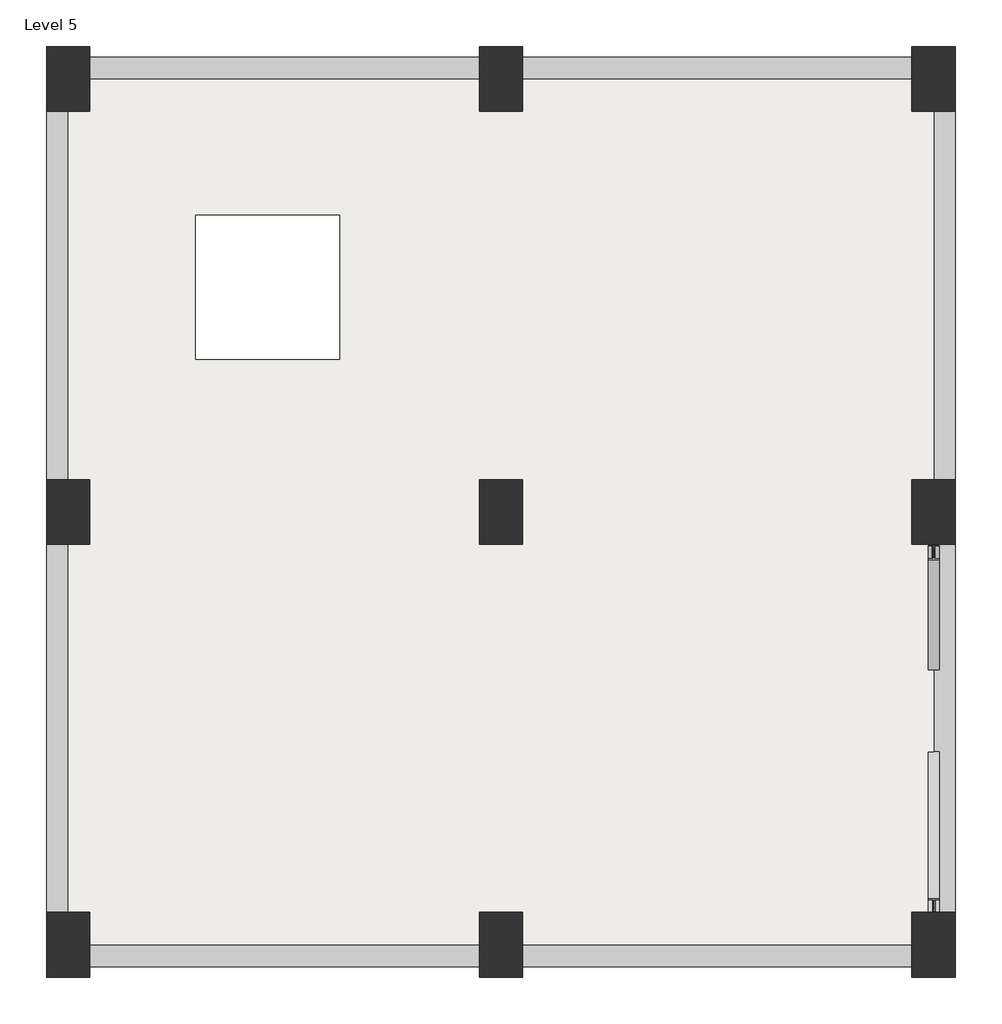
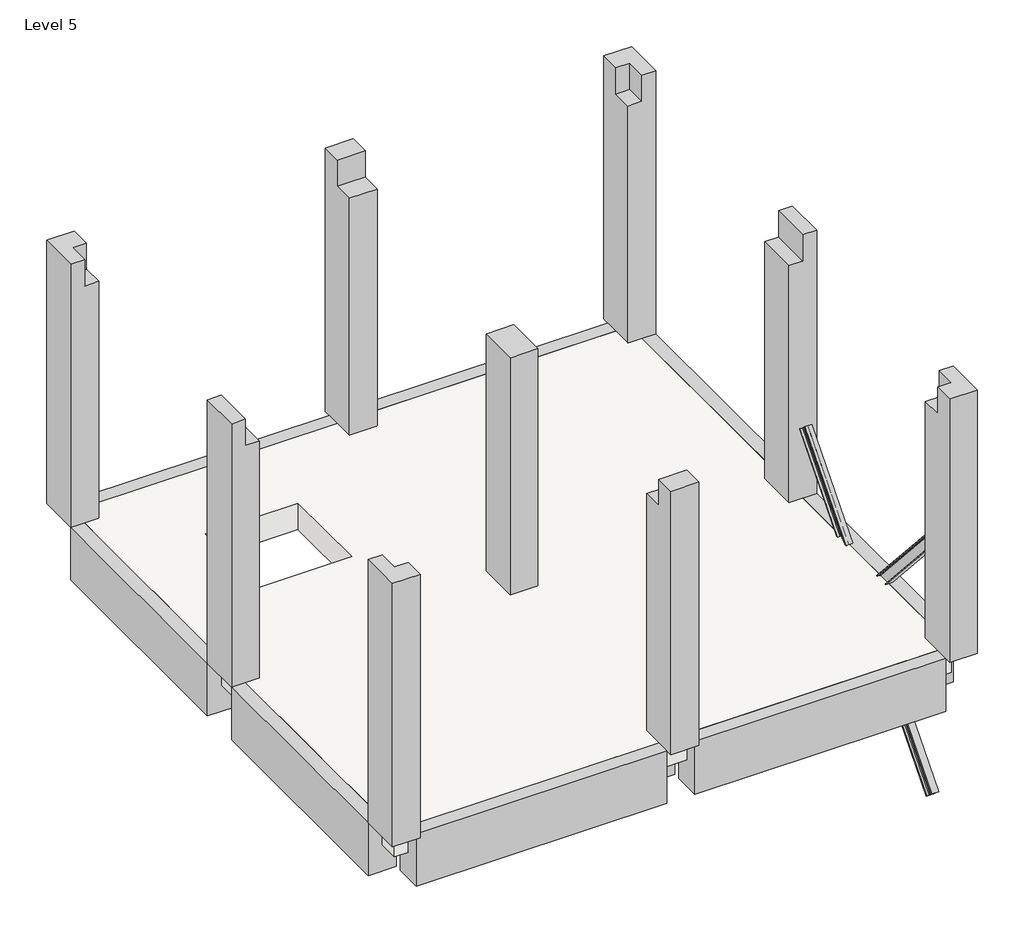
# One storey: 9 columns, 6 beams, 2 members, 1 slab.
"""IFC4 building model written with IfcOpenShell, lengths in millimetres."""

from ifc_helpers import new_model, si_unit, frame, origin, place, context, project, spatial, polyline, outline, extrude, faceted_brep, transform, mapped, element, save
from components import ub_universal_beams_ub127x76x13_58dc6553, ub_universal_beams_ub127x76x13_03bf5c3b

model = new_model("IFC4")

# Units and contexts
model_context = context("Model", 3, world=origin())
ifc_project = project(units=[si_unit("LENGTHUNIT", "METRE", prefix="MILLI")], contexts=[model_context])

# Site, building, storey
site = spatial("IfcSite", under=ifc_project)
building = spatial("IfcBuilding", under=site)
storey = spatial("IfcBuildingStorey", under=building, Name="Level 5", Elevation=12000.0)

# Beams
placement = place(None, origin())
element("IfcBeam", 1, ObjectType="Concrete-Rectangular Beam : 300 x 600mm", at=placement, inside=storey, context=model_context, shape_type="SweptSolid", body=[
    extrude(outline(polyline([(526.3372902, 11400.0), (226.3372902, 11400.0), (226.3372902, 11700.0), (376.3372902, 11700.0), (376.3372902, 12000.0), (526.3372902, 12000.0), (526.3372902, 11400.0)])), frame((2068.7595868, 0.0, 0.0), z_axis=(1.0, 0.0, 0.0), x_axis=(0.0, 1.0, 0.0)), (0.0, 0.0, 1.0), 2700.0),
    extrude(outline(polyline([(526.3372902, 11400.0), (226.3372902, 11400.0), (226.3372902, 11700.0), (376.3372902, 11700.0), (376.3372902, 12000.0), (526.3372902, 12000.0), (526.3372902, 11400.0)])), frame((-931.2404132, 0.0, 0.0), z_axis=(1.0, 0.0, 0.0), x_axis=(0.0, 1.0, 0.0)), (0.0, 0.0, 1.0), 2700.0),
])
element("IfcBeam", 2, ObjectType="Concrete-Rectangular Beam : 300 x 600mm", at=placement, inside=storey, context=model_context, shape_type="SweptSolid", body=[
    extrude(outline(polyline([(11400.0, 5068.7595868), (12000.0, 5068.7595868), (12000.0, 4918.7595868), (11700.0, 4918.7595868), (11700.0, 4768.7595868), (11400.0, 4768.7595868), (11400.0, 5068.7595868)])), frame((0.0, -2398.6627098, 0.0), z_axis=(0.0, 1.0, 0.0), x_axis=(0.0, 0.0, 1.0)), (0.0, 0.0, 1.0), 2550.0),
    extrude(outline(polyline([(11400.0, 5068.7595868), (12000.0, 5068.7595868), (12000.0, 4918.7595868), (11700.0, 4918.7595868), (11700.0, 4768.7595868), (11400.0, 4768.7595868), (11400.0, 5068.7595868)])), frame((0.0, -5398.6627098, 0.0), z_axis=(0.0, 1.0, 0.0), x_axis=(0.0, 0.0, 1.0)), (0.0, 0.0, 1.0), 2550.0),
])
element("IfcBeam", 3, ObjectType="Concrete-Rectangular Beam : 300 x 600mm", at=placement, inside=storey, context=model_context, shape_type="SweptSolid", body=[
    extrude(outline(polyline([(-5773.6627098, 11400.0), (-5773.6627098, 12000.0), (-5623.6627098, 12000.0), (-5623.6627098, 11700.0), (-5473.6627098, 11700.0), (-5473.6627098, 11400.0), (-5773.6627098, 11400.0)])), frame((2068.7595868, 0.0, 0.0), z_axis=(1.0, 0.0, 0.0), x_axis=(0.0, 1.0, 0.0)), (0.0, 0.0, 1.0), 2700.0),
    extrude(outline(polyline([(-5773.6627098, 11400.0), (-5773.6627098, 12000.0), (-5623.6627098, 12000.0), (-5623.6627098, 11700.0), (-5473.6627098, 11700.0), (-5473.6627098, 11400.0), (-5773.6627098, 11400.0)])), frame((-931.2404132, 0.0, 0.0), z_axis=(1.0, 0.0, 0.0), x_axis=(0.0, 1.0, 0.0)), (0.0, 0.0, 1.0), 2700.0),
])
element("IfcBeam", 4, ObjectType="Concrete-Rectangular Beam : 300 x 600mm", at=placement, inside=storey, context=model_context, shape_type="SweptSolid", body=[
    extrude(outline(polyline([(12000.0, -1231.2404132), (11400.0, -1231.2404132), (11400.0, -931.2404132), (11700.0, -931.2404132), (11700.0, -1081.2404132), (12000.0, -1081.2404132), (12000.0, -1231.2404132)])), frame((0.0, -5398.6627098, 0.0), z_axis=(0.0, 1.0, 0.0), x_axis=(0.0, 0.0, 1.0)), (0.0, 0.0, 1.0), 2550.0),
    extrude(outline(polyline([(12000.0, -1231.2404132), (11400.0, -1231.2404132), (11400.0, -931.2404132), (11700.0, -931.2404132), (11700.0, -1081.2404132), (12000.0, -1081.2404132), (12000.0, -1231.2404132)])), frame((0.0, -2398.6627098, 0.0), z_axis=(0.0, 1.0, 0.0), x_axis=(0.0, 0.0, 1.0)), (0.0, 0.0, 1.0), 2550.0),
])
element("IfcBeam", 5, ObjectType="Concrete-Rectangular Beam : 300 x 600mm", at=placement, inside=storey, context=model_context, shape_type="SweptSolid", body=[
    extrude(outline(polyline([(2068.7595868, -5398.6627098), (1768.7595868, -5398.6627098), (1768.7595868, -2848.6627098), (2068.7595868, -2848.6627098), (2068.7595868, -5398.6627098)])), frame((0.0, 0.0, 11400.0), z_axis=(0.0, 0.0, 1.0), x_axis=(1.0, 0.0, 0.0)), (0.0, 0.0, 1.0), 300.0),
    extrude(outline(polyline([(1768.7595868, 151.3372902), (2068.7595868, 151.3372902), (2068.7595868, -2398.6627098), (1768.7595868, -2398.6627098), (1768.7595868, 151.3372902)])), frame((0.0, 0.0, 11400.0), z_axis=(0.0, 0.0, 1.0), x_axis=(1.0, 0.0, 0.0)), (0.0, 0.0, 1.0), 300.0),
])
element("IfcBeam", 6, ObjectType="Concrete-Rectangular Beam : 300 x 600mm", at=placement, inside=storey, context=model_context, shape_type="SweptSolid", body=[
    extrude(outline(polyline([(4768.7595868, -2473.6627098), (4768.7595868, -2773.6627098), (2068.7595868, -2773.6627098), (2068.7595868, -2473.6627098), (4768.7595868, -2473.6627098)])), frame((0.0, 0.0, 11400.0), z_axis=(0.0, 0.0, 1.0), x_axis=(1.0, 0.0, 0.0)), (0.0, 0.0, 1.0), 300.0),
    extrude(outline(polyline([(-931.2404132, -2773.6627098), (-931.2404132, -2473.6627098), (1768.7595868, -2473.6627098), (1768.7595868, -2773.6627098), (-931.2404132, -2773.6627098)])), frame((0.0, 0.0, 11400.0), z_axis=(0.0, 0.0, 1.0), x_axis=(1.0, 0.0, 0.0)), (0.0, 0.0, 1.0), 300.0),
])

# Columns
element("IfcColumn", 7, ObjectType="Concrete-Rectangular-Column : 300 x 450mm", at=placement, inside=storey, context=model_context, shape_type="Brep", body=[
    faceted_brep([(-1231.2404132, -5848.6627098, 15000.0), (-931.2404132, -5848.6627098, 15000.0), (-931.2404132, -5623.6627098, 15000.0), (-1081.2404132, -5623.6627098, 15000.0), (-1081.2404132, -5398.6627098, 15000.0), (-1231.2404132, -5398.6627098, 15000.0), (-1231.2404132, -5848.6627098, 12000.0), (-1231.2404132, -5398.6627098, 12000.0), (-931.2404132, -5398.6627098, 12000.0), (-931.2404132, -5848.6627098, 12000.0), (-931.2404132, -5398.6627098, 14700.0), (-931.2404132, -5623.6627098, 14700.0), (-1081.2404132, -5398.6627098, 14700.0), (-1081.2404132, -5623.6627098, 14700.0)], [[[0, 1, 2, 3, 4, 5]], [[6, 7, 8, 9]], [[1, 0, 6, 9]], [[9, 8, 10, 11, 2, 1]], [[8, 7, 5, 4, 12, 10]], [[0, 5, 7, 6]], [[12, 13, 11, 10]], [[13, 3, 2, 11]], [[3, 13, 12, 4]]]),
])
element("IfcColumn", 8, ObjectType="Concrete-Rectangular-Column : 300 x 450mm", at=placement, inside=storey, context=model_context, shape_type="Brep", body=[
    faceted_brep([(1768.7595868, -5848.6627098, 15000.0), (2068.7595868, -5848.6627098, 15000.0), (2068.7595868, -5773.6627098, 15000.0), (2068.7595868, -5623.6627098, 15000.0), (1768.7595868, -5623.6627098, 15000.0), (1768.7595868, -5773.6627098, 15000.0), (1768.7595868, -5848.6627098, 12000.0), (1768.7595868, -5398.6627098, 12000.0), (2068.7595868, -5398.6627098, 12000.0), (2068.7595868, -5848.6627098, 12000.0), (2068.7595868, -5398.6627098, 14700.0), (2068.7595868, -5473.6627098, 14700.0), (2068.7595868, -5623.6627098, 14700.0), (1768.7595868, -5398.6627098, 14700.0), (1768.7595868, -5623.6627098, 14700.0), (1768.7595868, -5473.6627098, 14700.0)], [[[0, 1, 2, 3, 4, 5]], [[6, 7, 8, 9]], [[1, 0, 6, 9]], [[9, 8, 10, 11, 12, 3, 2, 1]], [[8, 7, 13, 10]], [[7, 6, 0, 5, 4, 14, 15, 13]], [[14, 12, 11, 10, 13, 15]], [[12, 14, 4, 3]]]),
])
element("IfcColumn", 9, ObjectType="Concrete-Rectangular-Column : 300 x 450mm", at=placement, inside=storey, context=model_context, shape_type="Brep", body=[
    faceted_brep([(4768.7595868, -5848.6627098, 15000.0), (5068.7595868, -5848.6627098, 15000.0), (5068.7595868, -5398.6627098, 15000.0), (4918.7595868, -5398.6627098, 15000.0), (4918.7595868, -5623.6627098, 15000.0), (4768.7595868, -5623.6627098, 15000.0), (4768.7595868, -5848.6627098, 12000.0), (4768.7595868, -5398.6627098, 12000.0), (5068.7595868, -5398.6627098, 12000.0), (5068.7595868, -5848.6627098, 12000.0), (4768.7595868, -5398.6627098, 14700.0), (4918.7595868, -5398.6627098, 14700.0), (4768.7595868, -5623.6627098, 14700.0), (4918.7595868, -5623.6627098, 14700.0)], [[[0, 1, 2, 3, 4, 5]], [[6, 7, 8, 9]], [[1, 0, 6, 9]], [[2, 1, 9, 8]], [[8, 7, 10, 11, 3, 2]], [[7, 6, 0, 5, 12, 10]], [[12, 13, 11, 10]], [[13, 4, 3, 11]], [[4, 13, 12, 5]]]),
])
element("IfcColumn", 10, ObjectType="Concrete-Rectangular-Column : 300 x 450mm", at=placement, inside=storey, context=model_context, shape_type="Brep", body=[
    faceted_brep([(-1231.2404132, -2398.6627098, 15000.0), (-1231.2404132, -2848.6627098, 15000.0), (-1081.2404132, -2848.6627098, 15000.0), (-1081.2404132, -2398.6627098, 15000.0), (-1231.2404132, -2848.6627098, 12000.0), (-1231.2404132, -2398.6627098, 12000.0), (-931.2404132, -2398.6627098, 12000.0), (-931.2404132, -2848.6627098, 12000.0), (-931.2404132, -2848.6627098, 14400.0), (-931.2404132, -2848.6627098, 14700.0), (-1081.2404132, -2848.6627098, 14700.0), (-1231.2404132, -2848.6627098, 14400.0), (-931.2404132, -2398.6627098, 14400.0), (-931.2404132, -2398.6627098, 14700.0), (-1231.2404132, -2398.6627098, 14400.0), (-1081.2404132, -2398.6627098, 14700.0)], [[[0, 1, 2, 3]], [[4, 5, 6, 7]], [[4, 7, 8, 9, 10, 2, 1, 11]], [[7, 6, 12, 13, 9, 8]], [[6, 5, 14, 0, 3, 15, 13, 12]], [[1, 0, 14, 5, 4, 11]], [[15, 10, 9, 13]], [[10, 15, 3, 2]]]),
])
element("IfcColumn", 11, ObjectType="Concrete-Rectangular-Column : 300 x 450mm", at=placement, inside=storey, context=model_context, shape_type="Brep", body=[
    faceted_brep([(1768.7595868, -2848.6627098, 12000.0), (1768.7595868, -2398.6627098, 12000.0), (2068.7595868, -2398.6627098, 12000.0), (2068.7595868, -2848.6627098, 12000.0), (2068.7595868, -2848.6627098, 14400.0), (2068.7595868, -2848.6627098, 14700.0), (1768.7595868, -2848.6627098, 14700.0), (1768.7595868, -2848.6627098, 14400.0), (2068.7595868, -2398.6627098, 14400.0), (2068.7595868, -2398.6627098, 14700.0), (2068.7595868, -2473.6627098, 14700.0), (2068.7595868, -2773.6627098, 14700.0), (1768.7595868, -2398.6627098, 14400.0), (1768.7595868, -2398.6627098, 14700.0), (1768.7595868, -2773.6627098, 14700.0), (1768.7595868, -2473.6627098, 14700.0)], [[[0, 1, 2, 3]], [[0, 3, 4, 5, 6, 7]], [[3, 2, 8, 9, 10, 11, 5, 4]], [[2, 1, 12, 13, 9, 8]], [[1, 0, 7, 6, 14, 15, 13, 12]], [[6, 5, 11, 10, 9, 13, 15, 14]]]),
])
element("IfcColumn", 12, ObjectType="Concrete-Rectangular-Column : 300 x 450mm", at=placement, inside=storey, context=model_context, shape_type="Brep", body=[
    faceted_brep([(5068.7595868, -2848.6627098, 15000.0), (5068.7595868, -2398.6627098, 15000.0), (4918.7595868, -2398.6627098, 15000.0), (4918.7595868, -2848.6627098, 15000.0), (4768.7595868, -2848.6627098, 12000.0), (4768.7595868, -2398.6627098, 12000.0), (5068.7595868, -2398.6627098, 12000.0), (5068.7595868, -2848.6627098, 12000.0), (5068.7595868, -2848.6627098, 14400.0), (4918.7595868, -2848.6627098, 14700.0), (4768.7595868, -2848.6627098, 14700.0), (4768.7595868, -2848.6627098, 14400.0), (5068.7595868, -2398.6627098, 14400.0), (4768.7595868, -2398.6627098, 14400.0), (4768.7595868, -2398.6627098, 14700.0), (4918.7595868, -2398.6627098, 14700.0)], [[[0, 1, 2, 3]], [[4, 5, 6, 7]], [[4, 7, 8, 0, 3, 9, 10, 11]], [[1, 0, 8, 7, 6, 12]], [[6, 5, 13, 14, 15, 2, 1, 12]], [[5, 4, 11, 10, 14, 13]], [[9, 15, 14, 10]], [[15, 9, 3, 2]]]),
])
element("IfcColumn", 13, ObjectType="Concrete-Rectangular-Column : 300 x 450mm", at=placement, inside=storey, context=model_context, shape_type="Brep", body=[
    faceted_brep([(-931.2404132, 601.3372902, 15000.0), (-1231.2404132, 601.3372902, 15000.0), (-1231.2404132, 151.3372902, 15000.0), (-1081.2404132, 151.3372902, 15000.0), (-1081.2404132, 376.3372902, 15000.0), (-931.2404132, 376.3372902, 15000.0), (-1231.2404132, 151.3372902, 12000.0), (-1231.2404132, 601.3372902, 12000.0), (-931.2404132, 601.3372902, 12000.0), (-931.2404132, 151.3372902, 12000.0), (-931.2404132, 151.3372902, 14700.0), (-1081.2404132, 151.3372902, 14700.0), (-931.2404132, 376.3372902, 14700.0), (-1081.2404132, 376.3372902, 14700.0)], [[[0, 1, 2, 3, 4, 5]], [[6, 7, 8, 9]], [[6, 9, 10, 11, 3, 2]], [[9, 8, 0, 5, 12, 10]], [[1, 0, 8, 7]], [[2, 1, 7, 6]], [[12, 13, 11, 10]], [[13, 4, 3, 11]], [[4, 13, 12, 5]]]),
])
element("IfcColumn", 14, ObjectType="Concrete-Rectangular-Column : 300 x 450mm", at=placement, inside=storey, context=model_context, shape_type="Brep", body=[
    faceted_brep([(2068.7595868, 601.3372902, 15000.0), (1768.7595868, 601.3372902, 15000.0), (1768.7595868, 526.3372902, 15000.0), (1768.7595868, 376.3372902, 15000.0), (2068.7595868, 376.3372902, 15000.0), (2068.7595868, 526.3372902, 15000.0), (1768.7595868, 151.3372902, 12000.0), (1768.7595868, 601.3372902, 12000.0), (2068.7595868, 601.3372902, 12000.0), (2068.7595868, 151.3372902, 12000.0), (2068.7595868, 151.3372902, 14700.0), (1768.7595868, 151.3372902, 14700.0), (2068.7595868, 376.3372902, 14700.0), (2068.7595868, 226.3372902, 14700.0), (1768.7595868, 226.3372902, 14700.0), (1768.7595868, 376.3372902, 14700.0)], [[[0, 1, 2, 3, 4, 5]], [[6, 7, 8, 9]], [[6, 9, 10, 11]], [[9, 8, 0, 5, 4, 12, 13, 10]], [[1, 0, 8, 7]], [[7, 6, 11, 14, 15, 3, 2, 1]], [[12, 15, 14, 11, 10, 13]], [[15, 12, 4, 3]]]),
])
element("IfcColumn", 15, ObjectType="Concrete-Rectangular-Column : 300 x 450mm", at=placement, inside=storey, context=model_context, shape_type="Brep", body=[
    faceted_brep([(5068.7595868, 151.3372902, 15000.0), (5068.7595868, 601.3372902, 15000.0), (4768.7595868, 601.3372902, 15000.0), (4768.7595868, 376.3372902, 15000.0), (4918.7595868, 376.3372902, 15000.0), (4918.7595868, 151.3372902, 15000.0), (4768.7595868, 151.3372902, 12000.0), (4768.7595868, 601.3372902, 12000.0), (5068.7595868, 601.3372902, 12000.0), (5068.7595868, 151.3372902, 12000.0), (4918.7595868, 151.3372902, 14700.0), (4768.7595868, 151.3372902, 14700.0), (4768.7595868, 376.3372902, 14700.0), (4918.7595868, 376.3372902, 14700.0)], [[[0, 1, 2, 3, 4, 5]], [[6, 7, 8, 9]], [[6, 9, 0, 5, 10, 11]], [[1, 0, 9, 8]], [[2, 1, 8, 7]], [[7, 6, 11, 12, 3, 2]], [[13, 12, 11, 10]], [[4, 13, 10, 5]], [[13, 4, 3, 12]]]),
])

# Members
ub_universal_beams_ub127x76x13_shape = ub_universal_beams_ub127x76x13_58dc6553(model_context)
element("IfcMember", 16, ObjectType="UB-Universal Beams : UB127x76x13", at=placement, inside=storey, context=model_context, shape_type="MappedRepresentation", body=[
    mapped(ub_universal_beams_ub127x76x13_shape, transform((4918.7595868, -3987.3365723, 11570.50801), x_axis=(0.0, 0.665487731700438, -0.7464087881022075), y_axis=(-1.0, 0.0, 0.0), z_axis=(0.0, 0.7464087881022075, 0.665487731700438))),
])
ub_universal_beams_ub127x76x13_2_shape = ub_universal_beams_ub127x76x13_03bf5c3b(model_context)
element("IfcMember", 17, ObjectType="UB-Universal Beams : UB127x76x13", at=placement, inside=storey, context=model_context, shape_type="MappedRepresentation", body=[
    mapped(ub_universal_beams_ub127x76x13_2_shape, transform((4918.7595868, -3946.516498, 11638.3225347), x_axis=(0.0, -0.652009917674905, -0.7582104373151055), y_axis=(1.0, 0.0, 0.0), z_axis=(0.0, -0.7582104373151055, 0.652009917674905))),
])

# Slab
element("IfcSlab", 18, ObjectType="Generic 300mm", at=placement, inside=storey, context=model_context, shape_type="Brep", body=[
    faceted_brep([(4918.7595868, 376.3372902, 11700.0), (4918.7595868, 151.3372902, 11700.0), (4918.7595868, -2398.6627098, 11700.0), (4918.7595868, -2848.6627098, 11700.0), (4918.7595868, -5398.6627098, 11700.0), (4918.7595868, -5623.6627098, 11700.0), (4768.7595868, -5623.6627098, 11700.0), (2068.7595868, -5623.6627098, 11700.0), (1768.7595868, -5623.6627098, 11700.0), (-931.2404132, -5623.6627098, 11700.0), (-1081.2404132, -5623.6627098, 11700.0), (-1081.2404132, -5398.6627098, 11700.0), (-1081.2404132, -2848.6627098, 11700.0), (-1081.2404132, -2398.6627098, 11700.0), (-1081.2404132, 151.3372902, 11700.0), (-1081.2404132, 376.3372902, 11700.0), (-931.2404132, 376.3372902, 11700.0), (1768.7595868, 376.3372902, 11700.0), (2068.7595868, 376.3372902, 11700.0), (4768.7595868, 376.3372902, 11700.0), (-198.5229478, -1566.5574371, 11700.0), (801.4770522, -1566.5574371, 11700.0), (801.4770522, -566.5574371, 11700.0), (-198.5229478, -566.5574371, 11700.0), (4918.7595868, -5623.6627098, 12000.0), (4918.7595868, -5398.6627098, 12000.0), (4918.7595868, -2848.6627098, 12000.0), (4918.7595868, -2398.6627098, 12000.0), (4918.7595868, 151.3372902, 12000.0), (4918.7595868, 376.3372902, 12000.0), (4768.7595868, 376.3372902, 12000.0), (2068.7595868, 376.3372902, 12000.0), (1768.7595868, 376.3372902, 12000.0), (-931.2404132, 376.3372902, 12000.0), (-1081.2404132, 376.3372902, 12000.0), (-1081.2404132, 151.3372902, 12000.0), (-1081.2404132, -2398.6627098, 12000.0), (-1081.2404132, -2848.6627098, 12000.0), (-1081.2404132, -5398.6627098, 12000.0), (-1081.2404132, -5623.6627098, 12000.0), (-931.2404132, -5623.6627098, 12000.0), (1768.7595868, -5623.6627098, 12000.0), (2068.7595868, -5623.6627098, 12000.0), (4768.7595868, -5623.6627098, 12000.0), (801.4770522, -1566.5574371, 12000.0), (-198.5229478, -1566.5574371, 12000.0), (-198.5229478, -566.5574371, 12000.0), (801.4770522, -566.5574371, 12000.0)], [[[0, 1, 2, 3, 4, 5, 6, 7, 8, 9, 10, 11, 12, 13, 14, 15, 16, 17, 18, 19], [20, 21, 22, 23]], [[24, 25, 26, 27, 28, 29, 30, 31, 32, 33, 34, 35, 36, 37, 38, 39, 40, 41, 42, 43], [44, 45, 46, 47]], [[5, 4, 3, 2, 1, 0, 29, 28, 27, 26, 25, 24]], [[10, 9, 8, 7, 6, 5, 24, 43, 42, 41, 40, 39]], [[15, 14, 13, 12, 11, 10, 39, 38, 37, 36, 35, 34]], [[0, 19, 18, 17, 16, 15, 34, 33, 32, 31, 30, 29]], [[20, 45, 44, 21]], [[21, 44, 47, 22]], [[22, 47, 46, 23]], [[45, 20, 23, 46]]]),
])

save(model, "model.ifc")

# Revit data of these elements
# Type "Concrete-Rectangular Beam : 300 x 600mm"
#   Length [instance default] = 1.524 m
#   b = 0.3 m
#   h = 0.6 m
#   Structural Material [instance default] = Concrete, Cast-in-Place gray
#   Assembly Code = ""
# Type "Concrete-Rectangular-Column : 300 x 450mm"
#   b = 0.3 m
#   h = 0.45 m
#   Structural Material [instance default] = Concrete, Cast-in-Place gray
# Type "UB-Universal Beams : UB127x76x13"
#   Section Name Key = "UB127X76X13"
#   Width = 7.6 cm
#   Web Thickness = 0.4 cm
#   Web Fillet = 0.76 cm
#   Warping Constant = 2000.0 cm⁶
#   Torsional Moment of Inertia = 2.85 cm⁴
#   Section Area = 16.5 cm²
#   Plastic Modulus weak axis = 22.6 cm³
#   Plastic Modulus strong axis = 84.2 cm³
#   Nominal Weight = 13.00 kgf/m
#   Moment of Inertia weak axis = 55.70 cm⁴
#   Moment of Inertia strong axis = 473.00 cm⁴
#   Height = 12.7 cm
#   Flange Thickness = 0.76 cm
#   Elastic Modulus weak axis = 14.7 cm³
#   Elastic Modulus strong axis = 74.6 cm³
#   Centroid Vertical = 6.35 cm
#   Centroid Horizontal = 3.8 cm
#   Bolt Spacing = 4.0 cm
#   Length [instance default] = 1.5 m
#   Structural Material [instance default] = Metal - Steel 43-275
#   Type Comments = ""
#   Assembly Code = ""
# Type "Generic 300mm"
#   Function = 0
#   Layers, outside or top first: 0.3 m no material (function 1)
# Elements 1, 2, 3, 4, 5, 6 (IfcBeam, "Concrete-Rectangular Beam : 300 x 600mm")
#   Structural Material = Concrete, Cast-in-Place gray
#   Phase Created = New Construction
#   Materials on its faces: "Concrete, Cast-in-Place gray"
# Elements 7, 8, 9, 10, 11, 12, 13, 14, 15 (IfcColumn, "Concrete-Rectangular-Column : 300 x 450mm")
#   Structural Material = Concrete, Cast-in-Place gray
#   Phase Created = New Construction
#   Materials on its faces: "Concrete, Cast-in-Place gray"
# Elements 16, 17 (IfcMember, "UB-Universal Beams : UB127x76x13")
#   Structural Material = Metal - Steel 43-275
#   Phase Created = New Construction
#   Materials on its faces: "Metal - Steel 43-275"
# Element 18 (IfcSlab, "Generic 300mm")
#   Height Offset From Level = 0 m
#   built-in parameter 1001954 = 1
#   Phase Created = New Construction
#   Materials on its faces: "Default Floor"
# Materials
#   "Concrete, Cast-in-Place gray": class "Concrete", colour RGB 192 192 192, transparency 0, Description = "Cast-in-place concrete", Cost = 0
#   "Metal - Steel 43-275": class "Metal", colour RGB 247 247 247, transparency 0, Cost = 0
#   "Default Floor": colour RGB 127 127 127, transparency 0, Cost = 0
